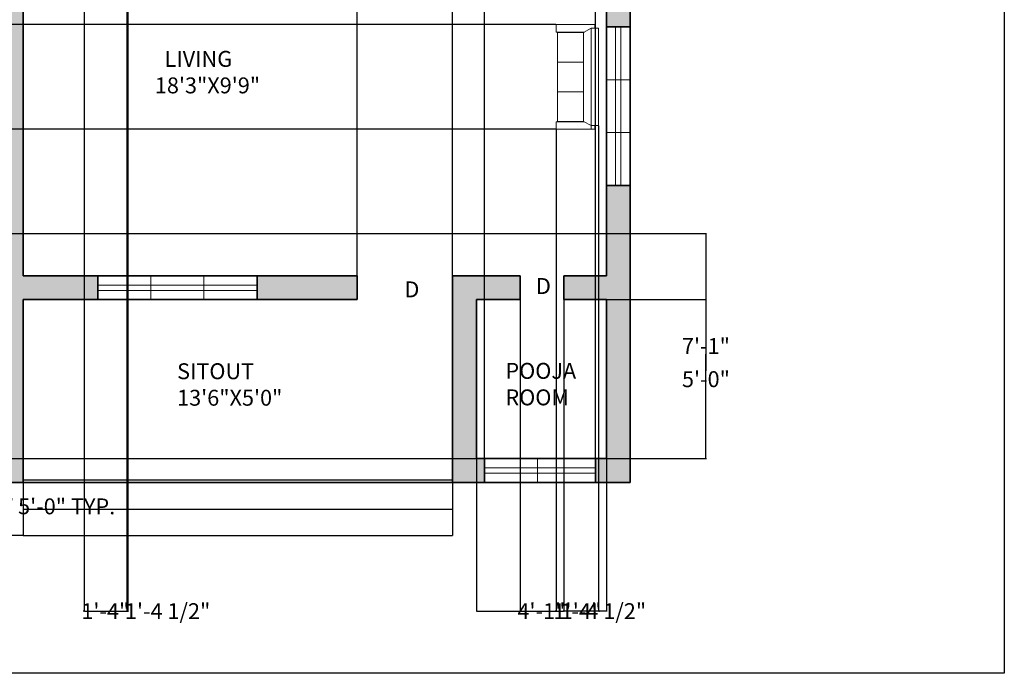
# Model space of a CAD drawing. Units: inches. Extents: x 2552 to 3196, y 4736 to 5443.
# Tile 3 of 8: x 2824 to 3196, y 4736 to 4983. Entities that reach past the tile are written whole.
import ezdxf

# ---------------------------------------------------------------- set-up
doc = ezdxf.new("R2010")
doc.units = ezdxf.units.IN
doc.header["$MEASUREMENT"] = 0
for name, color, linetype, lineweight in [('A-ANNO-DIMS', 2, 'Continuous', 18), ('A-ANNO-TTLB', 7, 'Continuous', 25), ('A-AREA-IDEN', 7, 'Continuous', 18), ('A-DOOR-IDEN', 7, 'Continuous', 18), ('A-FLOR-STRS', 7, 'Continuous', 25), ('A-FURN', 8, 'Continuous', 18), ('A-GLAZ', 4, 'Continuous', 18), ('A-WALL', 7, 'Continuous', 35)]:
    doc.layers.add(name, color=color, linetype=linetype, lineweight=lineweight)
doc.layers.add('A-WALL-PATT', color=30, linetype='Continuous', lineweight=13, true_color=0xf8991e)
doc.styles.get("Standard").update_dxf_attribs({"font": 'arial.ttf'})
doc.dimstyles.get("Standard").update_dxf_attribs({"dimtxt": 6, "dimasz": 0.18, "dimexe": 0.18, "dimexo": 0.0625, "dimgap": 0.09, "dimtad": 0, "dimtih": 1, "dimtoh": 1, "dimdec": 1, "dimzin": 0, "dimdsep": 46, "dimlunit": 3, "dimtxsty": 'Standard', "dimcen": 0.09, "dimadec": 0, "dimazin": 0, "dimtfac": 1, "dimtdec": 1, "dimtofl": 0, "dimtmove": 0, "dimatfit": 3, "dimfxl": 1, "dimtolj": 1, "dimtzin": 0, "dimarcsym": 0})

# ---------------------------------------------------------------- blocks, each defined once
blk = doc.blocks.new('WIN-60IN-THREE-LIGHT')
for p, q in [((60, 9), (0, 9)), ((20, 9), (20, 0)), ((40, 0), (40, 9)), ((60, 5.5), (0, 5.5)), ((0, 3.5), (60, 3.5)), ((0, 0), (60, 0))]:
    blk.add_line(p, q)
blk = doc.blocks.new('*D9')
at = {"layer": 'A-ANNO-DIMS', "color": 0, "lineweight": -2, "transparency": 16777216}
for p, q in [((2725.76, 4808.26), (2725.76, 4799.14)), ((2785.76, 4808.26), (2785.76, 4799.14)), ((2725.94, 4799.32), (2785.58, 4799.32)), ((2785.76, 4799.32), (2785.94, 4799.32))]:
    blk.add_line(p, q, dxfattribs=at)
at = {"layer": 'A-ANNO-DIMS', "color": 0, "transparency": 16777216}
for points in [[(2725.94, 4799.35), (2725.94, 4799.29), (2725.76, 4799.32)], [(2785.58, 4799.35), (2785.58, 4799.29), (2785.76, 4799.32)]]:
    blk.add_solid(points, dxfattribs=at)
at = {"layer": 'Defpoints', "color": 0, "transparency": 16777216}
for p in [(2725.76, 4808.32), (2785.76, 4808.32), (2785.76, 4799.32)]:
    blk.add_point(p, dxfattribs=at)
at = {"layer": 'A-ANNO-DIMS', "color": 0, "transparency": 16777216, "insert": (2823.99, 4799.32), "char_height": 6, "attachment_point": 5}
blk.add_mtext('\\A1;WINDOW 5\'-0" TYP.', dxfattribs=at)
blk = doc.blocks.new('*D21')
at = {"layer": 'A-ANNO-DIMS', "color": 0, "lineweight": -2, "transparency": 16777216}
for p, q in [((2996.66, 4817.26), (2996.66, 4759.59)), ((3045.66, 4817.26), (3045.66, 4759.59)), ((2996.84, 4759.77), (3012.97, 4759.77)), ((3045.48, 4759.77), (3029.34, 4759.77))]:
    blk.add_line(p, q, dxfattribs=at)
at = {"layer": 'A-ANNO-DIMS', "color": 0, "transparency": 16777216}
for points in [[(2996.84, 4759.8), (2996.84, 4759.74), (2996.66, 4759.77)], [(3045.48, 4759.8), (3045.48, 4759.74), (3045.66, 4759.77)]]:
    blk.add_solid(points, dxfattribs=at)
at = {"layer": 'Defpoints', "color": 0, "transparency": 16777216}
for p in [(2996.66, 4817.32), (3045.66, 4817.32), (3045.66, 4759.77)]:
    blk.add_point(p, dxfattribs=at)
at = {"layer": 'A-ANNO-DIMS', "color": 0, "transparency": 16777216, "insert": (3021.16, 4759.77), "char_height": 6, "attachment_point": 5}
blk.add_mtext('\\A1;4\'-1"', dxfattribs=at)
blk = doc.blocks.new('*D22')
at = {"layer": 'A-ANNO-DIMS', "color": 0, "lineweight": -2, "transparency": 16777216}
for p, q in [((3045.72, 4877.32), (3083.39, 4877.32)), ((3083.21, 4877.14), (3083.21, 4850.47)), ((3083.21, 4817.5), (3083.21, 4844.16)), ((3045.72, 4817.32), (3083.39, 4817.32))]:
    blk.add_line(p, q, dxfattribs=at)
at = {"layer": 'A-ANNO-DIMS', "color": 0, "transparency": 16777216}
for points in [[(3083.18, 4877.14), (3083.24, 4877.14), (3083.21, 4877.32)], [(3083.18, 4817.5), (3083.24, 4817.5), (3083.21, 4817.32)]]:
    blk.add_solid(points, dxfattribs=at)
at = {"layer": 'Defpoints', "color": 0, "transparency": 16777216}
for p in [(3045.66, 4877.32), (3083.21, 4877.32), (3045.66, 4817.32)]:
    blk.add_point(p, dxfattribs=at)
at = {"layer": 'A-ANNO-DIMS', "color": 0, "transparency": 16777216, "insert": (3083.21, 4847.32), "char_height": 6, "attachment_point": 5}
blk.add_mtext('\\A1;5\'-0"', dxfattribs=at)
blk = doc.blocks.new('*D23')
at = {"layer": 'A-ANNO-DIMS', "color": 0, "lineweight": -2, "transparency": 16777216}
for p, q in [((2825.59, 4808.32), (2662.93, 4808.32)), ((2663.11, 4808.14), (2663.11, 4801.47)), ((2663.11, 4788.5), (2663.11, 4795.16)), ((2825.59, 4788.32), (2662.93, 4788.32))]:
    blk.add_line(p, q, dxfattribs=at)
at = {"layer": 'A-ANNO-DIMS', "color": 0, "transparency": 16777216}
for points in [[(2663.08, 4808.14), (2663.14, 4808.14), (2663.11, 4808.32)], [(2663.08, 4788.5), (2663.14, 4788.5), (2663.11, 4788.32)]]:
    blk.add_solid(points, dxfattribs=at)
at = {"layer": 'Defpoints', "color": 0, "transparency": 16777216}
for p in [(2663.11, 4808.32), (2825.66, 4808.32), (2825.66, 4788.32)]:
    blk.add_point(p, dxfattribs=at)
at = {"layer": 'A-ANNO-DIMS', "color": 0, "transparency": 16777216, "insert": (2663.11, 4798.32), "char_height": 6, "attachment_point": 5}
blk.add_mtext('\\A1;1\'-8"', dxfattribs=at)
blk = doc.blocks.new('*D24')
at = {"layer": 'A-ANNO-DIMS', "color": 0, "lineweight": -2, "transparency": 16777216}
for p, q in [((2951.66, 4886.38), (2951.66, 5320.05)), ((2951.84, 5319.87), (2961.59, 5319.87)), ((2987.48, 5319.87), (2977.72, 5319.87)), ((2987.66, 4886.38), (2987.66, 5320.05))]:
    blk.add_line(p, q, dxfattribs=at)
at = {"layer": 'A-ANNO-DIMS', "color": 0, "transparency": 16777216}
for points in [[(2951.84, 5319.9), (2951.84, 5319.84), (2951.66, 5319.87)], [(2987.48, 5319.9), (2987.48, 5319.84), (2987.66, 5319.87)]]:
    blk.add_solid(points, dxfattribs=at)
at = {"layer": 'Defpoints', "color": 0, "transparency": 16777216}
for p in [(2987.66, 5319.87), (2951.66, 4886.32), (2987.66, 4886.32)]:
    blk.add_point(p, dxfattribs=at)
at = {"layer": 'A-ANNO-DIMS', "color": 0, "transparency": 16777216, "insert": (2969.66, 5319.87), "char_height": 6, "attachment_point": 5}
blk.add_mtext('\\A1;3\'-0"', dxfattribs=at)
blk = doc.blocks.new('*D25')
at = {"layer": 'A-ANNO-DIMS', "color": 0, "lineweight": -2, "transparency": 16777216}
for p, q in [((3013.11, 4877.26), (3013.11, 4759.59)), ((3029.6, 4877.26), (3029.6, 4759.59)), ((3013.29, 4759.77), (3029.42, 4759.77)), ((3029.6, 4759.77), (3029.78, 4759.77))]:
    blk.add_line(p, q, dxfattribs=at)
at = {"layer": 'A-ANNO-DIMS', "color": 0, "transparency": 16777216}
for points in [[(3013.29, 4759.8), (3013.29, 4759.74), (3013.11, 4759.77)], [(3029.42, 4759.8), (3029.42, 4759.74), (3029.6, 4759.77)]]:
    blk.add_solid(points, dxfattribs=at)
at = {"layer": 'Defpoints', "color": 0, "transparency": 16777216}
for p in [(3013.11, 4877.32), (3029.6, 4877.32), (3029.6, 4759.77)]:
    blk.add_point(p, dxfattribs=at)
at = {"layer": 'A-ANNO-DIMS', "color": 0, "transparency": 16777216, "insert": (3044.56, 4759.77), "char_height": 6, "attachment_point": 5}
blk.add_mtext('\\A1;1\'-4 1/2"', dxfattribs=at)
blk = doc.blocks.new('*D27')
at = {"layer": 'A-ANNO-DIMS', "color": 0, "lineweight": -2, "transparency": 16777216}
for p, q in [((2999.73, 4817.38), (2999.73, 5320.05)), ((2999.91, 5319.87), (3012.6, 5319.87)), ((3041.41, 5319.87), (3028.73, 5319.87)), ((3041.59, 4817.38), (3041.59, 5320.05))]:
    blk.add_line(p, q, dxfattribs=at)
at = {"layer": 'A-ANNO-DIMS', "color": 0, "transparency": 16777216}
for points in [[(2999.91, 5319.9), (2999.91, 5319.84), (2999.73, 5319.87)], [(3041.41, 5319.9), (3041.41, 5319.84), (3041.59, 5319.87)]]:
    blk.add_solid(points, dxfattribs=at)
at = {"layer": 'Defpoints', "color": 0, "transparency": 16777216}
for p in [(3041.59, 5319.87), (2999.73, 4817.32), (3041.59, 4817.32)]:
    blk.add_point(p, dxfattribs=at)
at = {"layer": 'A-ANNO-DIMS', "color": 0, "transparency": 16777216, "insert": (3020.66, 5319.87), "char_height": 6, "attachment_point": 5}
blk.add_mtext('\\A1;3\'-6"', dxfattribs=at)
blk = doc.blocks.new('*D31')
at = {"layer": 'A-ANNO-DIMS', "color": 0, "lineweight": -2, "transparency": 16777216}
for p, q in [((2848.66, 5282.26), (2848.66, 4759.59)), ((2865.22, 5282.26), (2865.22, 4759.59)), ((2848.84, 4759.77), (2865.04, 4759.77)), ((2865.22, 4759.77), (2865.4, 4759.77))]:
    blk.add_line(p, q, dxfattribs=at)
at = {"layer": 'A-ANNO-DIMS', "color": 0, "transparency": 16777216}
for points in [[(2848.84, 4759.8), (2848.84, 4759.74), (2848.66, 4759.77)], [(2865.04, 4759.8), (2865.04, 4759.74), (2865.22, 4759.77)]]:
    blk.add_solid(points, dxfattribs=at)
at = {"layer": 'Defpoints', "color": 0, "transparency": 16777216}
for p in [(2848.66, 5282.32), (2865.22, 5282.32), (2865.22, 4759.77)]:
    blk.add_point(p, dxfattribs=at)
at = {"layer": 'A-ANNO-DIMS', "color": 0, "transparency": 16777216, "insert": (2880.18, 4759.77), "char_height": 6, "attachment_point": 5}
blk.add_mtext('\\A1;1\'-4 1/2"', dxfattribs=at)
blk = doc.blocks.new('*D32')
at = {"layer": 'A-ANNO-DIMS', "color": 0, "lineweight": -2, "transparency": 16777216}
for p, q in [((2864.75, 5194.1), (2864.75, 4759.59)), ((2848.66, 5191.26), (2848.66, 4759.59)), ((2848.48, 4759.77), (2848.3, 4759.77)), ((2864.93, 4759.77), (2865.11, 4759.77))]:
    blk.add_line(p, q, dxfattribs=at)
at = {"layer": 'A-ANNO-DIMS', "color": 0, "transparency": 16777216}
for points in [[(2848.48, 4759.8), (2848.48, 4759.74), (2848.66, 4759.77)], [(2864.93, 4759.8), (2864.93, 4759.74), (2864.75, 4759.77)]]:
    blk.add_solid(points, dxfattribs=at)
at = {"layer": 'Defpoints', "color": 0, "transparency": 16777216}
for p in [(2864.75, 5194.17), (2848.66, 5191.32), (2864.75, 4759.77)]:
    blk.add_point(p, dxfattribs=at)
at = {"layer": 'A-ANNO-DIMS', "color": 0, "transparency": 16777216, "insert": (2856.7, 4759.77), "char_height": 6, "attachment_point": 5}
blk.add_mtext('\\A1;1\'-4"', dxfattribs=at)
blk = doc.blocks.new('*D35')
at = {"layer": 'A-ANNO-DIMS', "color": 0, "lineweight": -2, "transparency": 16777216}
for p, q in [((3026.66, 4981.14), (2662.93, 4981.14)), ((2663.11, 4980.96), (2663.11, 4964.56)), ((2663.11, 4941.78), (2663.11, 4958.17)), ((3026.66, 4941.6), (2662.93, 4941.6))]:
    blk.add_line(p, q, dxfattribs=at)
at = {"layer": 'A-ANNO-DIMS', "color": 0, "transparency": 16777216}
for points in [[(2663.08, 4980.96), (2663.14, 4980.96), (2663.11, 4981.14)], [(2663.08, 4941.78), (2663.14, 4941.78), (2663.11, 4941.6)]]:
    blk.add_solid(points, dxfattribs=at)
at = {"layer": 'Defpoints', "color": 0, "transparency": 16777216}
for p in [(3026.72, 4981.14), (2663.11, 4941.6), (3026.72, 4941.6)]:
    blk.add_point(p, dxfattribs=at)
at = {"layer": 'A-ANNO-DIMS', "color": 0, "transparency": 16777216, "insert": (2663.11, 4961.37), "char_height": 6, "attachment_point": 5}
blk.add_mtext('\\A1;3\'-3 1/2"', dxfattribs=at)
blk = doc.blocks.new('*D36')
at = {"layer": 'A-ANNO-DIMS', "color": 0, "lineweight": -2, "transparency": 16777216}
for p, q in [((3042.69, 4942.94), (3042.69, 4759.59)), ((3026.72, 4941.53), (3026.72, 4759.59)), ((3026.54, 4759.77), (3026.36, 4759.77)), ((3042.87, 4759.77), (3043.05, 4759.77))]:
    blk.add_line(p, q, dxfattribs=at)
at = {"layer": 'A-ANNO-DIMS', "color": 0, "transparency": 16777216}
for points in [[(3026.54, 4759.8), (3026.54, 4759.74), (3026.72, 4759.77)], [(3042.87, 4759.8), (3042.87, 4759.74), (3042.69, 4759.77)]]:
    blk.add_solid(points, dxfattribs=at)
at = {"layer": 'Defpoints', "color": 0, "transparency": 16777216}
for p in [(3042.69, 4943.01), (3026.72, 4941.6), (3042.69, 4759.77)]:
    blk.add_point(p, dxfattribs=at)
at = {"layer": 'A-ANNO-DIMS', "color": 0, "transparency": 16777216, "insert": (3034.7, 4759.77), "char_height": 6, "attachment_point": 5}
blk.add_mtext('\\A1;1\'-4"', dxfattribs=at)
blk = doc.blocks.new('*D39')
at = {"layer": 'A-ANNO-DIMS', "color": 0, "lineweight": -2, "transparency": 16777216}
for p, q in [((2700.72, 4902.32), (3083.39, 4902.32)), ((3083.21, 4902.14), (3083.21, 4862.92)), ((3083.21, 4817.5), (3083.21, 4856.72)), ((2700.72, 4817.32), (3083.39, 4817.32))]:
    blk.add_line(p, q, dxfattribs=at)
at = {"layer": 'A-ANNO-DIMS', "color": 0, "transparency": 16777216}
for points in [[(3083.18, 4902.14), (3083.24, 4902.14), (3083.21, 4902.32)], [(3083.18, 4817.5), (3083.24, 4817.5), (3083.21, 4817.32)]]:
    blk.add_solid(points, dxfattribs=at)
at = {"layer": 'Defpoints', "color": 0, "transparency": 16777216}
for p in [(2700.66, 4902.32), (3083.21, 4902.32), (2700.66, 4817.32)]:
    blk.add_point(p, dxfattribs=at)
at = {"layer": 'A-ANNO-DIMS', "color": 0, "transparency": 16777216, "insert": (3083.21, 4859.82), "char_height": 6, "attachment_point": 5}
blk.add_mtext('\\A1;7\'-1"', dxfattribs=at)

msp = doc.modelspace()

# ---------------------------------------------------------------- hatches: boundary and pattern name
at = {"layer": 'A-WALL-PATT'}
h = msp.add_hatch(color=256, dxfattribs=at)
h.dxf.hatch_style = 1
h.paths.add_polyline_path([(2700.66, 5282.32), (2732.91, 5282.32), (2732.91, 5291.32), (2691.66, 5291.32), (2691.66, 5248.4), (2700.66, 5248.4)])
h.paths.add_polyline_path([(2865.22, 5291.32), (2792.91, 5291.32), (2792.91, 5282.32), (2839.66, 5282.32), (2839.66, 5136.32), (2848.66, 5136.32), (2848.66, 5182.32), (2913.66, 5182.32), (2913.66, 5246.32), (2904.66, 5246.32), (2904.66, 5191.32), (2848.66, 5191.32), (2848.66, 5282.32), (2865.22, 5282.32)])
h.paths.add_polyline_path([(2946.08, 5291.32), (2889.22, 5291.32), (2889.22, 5282.32), (2946.08, 5282.32)])
h.paths.add_polyline_path([(3054.66, 5291.32), (3006.08, 5291.32), (3006.08, 5282.32), (3045.66, 5282.32), (3045.66, 5249.18), (3054.66, 5249.18)])
h.paths.add_polyline_path([(3054.66, 5189.18), (3045.66, 5189.18), (3045.66, 5145.32), (2904.66, 5145.32), (2904.66, 5136.32), (3045.66, 5136.32), (3045.66, 5103.54), (3054.66, 5103.54)])
h.paths.add_polyline_path([(3054.66, 5043.54), (3045.66, 5043.54), (3045.66, 5012.32), (2913.66, 5012.32), (2913.66, 5100.32), (2904.66, 5100.32), (2904.66, 5003.32), (3045.66, 5003.32), (3045.66, 4980.34), (3054.66, 4980.34)])
h.paths.add_polyline_path([(3054.66, 4920.34), (3045.66, 4920.34), (3045.66, 4886.32), (3029.6, 4886.32), (3029.6, 4877.32), (3045.66, 4877.32), (3045.66, 4817.32), (3041.59, 4817.32), (3041.59, 4808.32), (3054.66, 4808.32)])
h.paths.add_polyline_path([(2996.66, 4877.32), (3013.11, 4877.32), (3013.11, 4886.32), (2987.66, 4886.32), (2987.66, 4808.32), (2999.73, 4808.32), (2999.73, 4817.32), (2996.66, 4817.32)])
h.paths.add_polyline_path([(2825.66, 4877.32), (2853.9, 4877.32), (2853.9, 4886.32), (2825.66, 4886.32), (2825.66, 5000.12), (2816.66, 5000.12), (2816.66, 4817.32), (2785.76, 4817.32), (2785.76, 4808.32), (2825.66, 4808.32)])
h.paths.add_polyline_path([(2951.66, 4886.32), (2913.9, 4886.32), (2913.9, 4877.32), (2951.66, 4877.32)])
h.paths.add_polyline_path([(2725.76, 4817.32), (2700.66, 4817.32), (2700.66, 4833.17), (2691.66, 4833.17), (2691.66, 4808.32), (2725.76, 4808.32)])
h.paths.add_polyline_path([(2700.66, 4902.32), (2691.66, 4902.32), (2691.66, 4869.17), (2700.66, 4869.17)])
h.paths.add_polyline_path([(2765.91, 4947.32), (2700.66, 4947.32), (2700.66, 4977.71), (2691.66, 4977.71), (2691.66, 4938.32), (2765.91, 4938.32)])
h.paths.add_polyline_path([(2825.66, 5077.32), (2773.66, 5077.32), (2773.66, 5112.32), (2764.66, 5112.32), (2764.66, 5077.32), (2700.66, 5077.32), (2700.66, 5102.51), (2691.66, 5102.51), (2691.66, 5037.71), (2700.66, 5037.71), (2700.66, 5068.32), (2816.66, 5068.32), (2816.66, 5036.12), (2825.66, 5036.12)])
h.paths.add_polyline_path([(2803.66, 5145.32), (2700.66, 5145.32), (2700.66, 5188.4), (2691.66, 5188.4), (2691.66, 5126.51), (2700.66, 5126.51), (2700.66, 5136.32), (2803.66, 5136.32)])

# ---------------------------------------------------------------- linework, layer by layer
at = {"layer": 'A-ANNO-TTLB'}
msp.add_lwpolyline([(2551.65, 5442.6), (3195.75, 5442.6), (3195.75, 4736.32), (2551.65, 4736.32)], close=True, dxfattribs=at)
at = {"layer": 'A-FLOR-STRS'}
for p, q in [((2825.66, 4809.32), (2987.66, 4809.32)), ((2825.66, 4808.32), (2987.66, 4808.32)), ((2825.66, 4808.32), (2825.66, 4788.32)), ((2987.66, 4808.32), (2987.66, 4788.32)), ((2825.66, 4798.32), (2987.66, 4798.32)), ((2825.66, 4788.32), (2987.66, 4788.32))]:
    msp.add_line(p, q, dxfattribs=at)
at = {"layer": 'A-FURN'}
for p, q in [((3041.28, 4981.14), (3026.72, 4981.14)), ((3026.72, 4978.32), (3026.72, 4981.14)), ((3041.28, 4979.73), (3041.28, 4981.14)), ((3037.45, 4978.32), (3026.72, 4978.32)), ((3037.05, 4978.14), (3039.87, 4979.73)), ((3039.87, 4941.6), (3039.87, 4979.73)), ((3039.87, 4979.73), (3042.69, 4979.73)), ((3042.69, 4943.01), (3042.69, 4979.73)), ((3027.19, 4966.96), (3037.05, 4966.96)), ((3027.19, 4955.78), (3037.05, 4955.78)), ((3037.27, 4944.42), (3026.72, 4944.42)), ((3026.72, 4944.42), (3026.72, 4941.6)), ((3027.19, 4944.59), (3037.05, 4944.59)), ((3039.87, 4943.01), (3037.05, 4944.59)), ((3039.87, 4943.01), (3042.69, 4943.01)), ((3041.28, 4941.6), (3041.28, 4943.01)), ((3041.28, 4941.6), (3026.72, 4941.6))]:
    msp.add_line(p, q, dxfattribs=at)
msp.add_lwpolyline([(3037.05, 4944.59), (3037.05, 4978.14), (3027.19, 4978.14), (3027.19, 4944.59)], dxfattribs=at)
at = {"layer": 'A-GLAZ'}
for p, q in [((2999.73, 4817.32), (3041.59, 4817.32)), ((3019.73, 4808.32), (3019.73, 4817.32)), ((2999.73, 4813.82), (3041.59, 4813.82)), ((3041.59, 4811.82), (2999.73, 4811.82)), ((3041.59, 4808.32), (2999.73, 4808.32))]:
    msp.add_line(p, q, dxfattribs=at)
at = {"layer": 'A-WALL'}
for p, q in [((3054.66, 5291.32), (3054.66, 4808.32)), ((3045.66, 5003.32), (3045.66, 4886.32)), ((2825.66, 5000.12), (2825.66, 4886.32)), ((3045.66, 4980.34), (3054.66, 4980.34)), ((3054.66, 4920.34), (3045.66, 4920.34)), ((2825.66, 4886.32), (2951.66, 4886.32)), ((2853.9, 4886.32), (2853.9, 4877.32)), ((2913.9, 4877.32), (2913.9, 4886.32)), ((2951.66, 4886.32), (2951.66, 4877.32)), ((2987.66, 4886.32), (2987.66, 4808.32)), ((2987.66, 4886.32), (3013.11, 4886.32)), ((3013.11, 4886.32), (3013.11, 4877.32)), ((3029.6, 4877.32), (3029.6, 4886.32)), ((3029.6, 4886.32), (3045.66, 4886.32)), ((2825.66, 4877.32), (2951.66, 4877.32)), ((2825.66, 4877.32), (2825.66, 4808.32)), ((2996.66, 4877.32), (2996.66, 4817.32)), ((2996.66, 4877.32), (3013.11, 4877.32)), ((3029.6, 4877.32), (3045.66, 4877.32)), ((3045.66, 4877.32), (3045.66, 4817.32)), ((2996.66, 4817.32), (3045.66, 4817.32)), ((2999.73, 4808.32), (2999.73, 4817.32)), ((3041.59, 4817.32), (3041.59, 4808.32)), ((2691.66, 4808.32), (3054.66, 4808.32))]:
    msp.add_line(p, q, dxfattribs=at)

# ---------------------------------------------------------------- block references
at = {"layer": 'A-GLAZ', "rotation": 89.99999999999903}
msp.add_blockref('WIN-60IN-THREE-LIGHT', (3054.66, 4920.34), dxfattribs=at)
at = {"layer": 'A-GLAZ'}
msp.add_blockref('WIN-60IN-THREE-LIGHT', (2853.9, 4877.32), dxfattribs=at)

# ---------------------------------------------------------------- texts
at = {"layer": 'A-AREA-IDEN', "char_height": 6, "attachment_point": 1}
for s, width, insert in [('  LIVING\\P18\'3"X9\'9"', 111.7207, (2875.36, 4971.18)), ('SITOUT\\P13\'6"X5\'0"', 93.2404, (2883.75, 4853.31)), ('POOJA\\PROOM', 44.4868, (3007.58, 4853.45))]:
    msp.add_mtext_dynamic_manual_height_columns(s, width=width, gutter_width=1, heights=[0], dxfattribs=dict(at, insert=insert))
at = {"layer": 'A-DOOR-IDEN', "char_height": 6, "attachment_point": 1}
for insert in [(2969.49, 4884.2), (3019.11, 4885.47)]:
    msp.add_mtext_dynamic_manual_height_columns('D', width=10.2167, gutter_width=1, heights=[0], dxfattribs=dict(at, insert=insert))

# ---------------------------------------------------------------- dimensions: what is measured, and where the dimension line sits
at = {"layer": 'A-ANNO-DIMS'}
for base, p1, p2, picture, middle in [((2987.66, 5319.87), (2951.66, 4886.32), (2987.66, 4886.32), '*D24', (2969.66, 5319.87)), ((3041.59, 5319.87), (2999.73, 4817.32), (3041.59, 4817.32), '*D27', (3020.66, 5319.87)), ((2865.22, 4759.77), (2848.66, 5282.32), (2865.22, 5282.32), '*D31', (2880.18, 4759.77)), ((2864.75, 4759.77), (2848.66, 5191.32), (2864.75, 5194.17), '*D32', (2856.7, 4759.77)), ((3042.69, 4759.77), (3026.72, 4941.6), (3042.69, 4943.01), '*D36', (3034.7, 4759.77)), ((3029.6, 4759.77), (3013.11, 4877.32), (3029.6, 4877.32), '*D25', (3044.56, 4759.77)), ((3045.66, 4759.77), (2996.66, 4817.32), (3045.66, 4817.32), '*D21', (3021.16, 4759.77))]:
    dim = msp.add_linear_dim(base=base, p1=p1, p2=p2, dimstyle='Standard', override={"dimdec": 1, "dimlfac": 1, "dimrnd": 0, "dimzin": 1, "dimdsep": 46, "dimlunit": 4, "dimfrac": 2}, dxfattribs=at)
    dim.commit()
    dim.dimension.update_dxf_attribs({"geometry": picture, "text_midpoint": middle})
for base, p1, p2, picture, middle in [((2663.11, 4941.6), (3026.72, 4981.14), (3026.72, 4941.6), '*D35', (2663.11, 4961.37)), ((3083.21, 4902.32), (2700.66, 4817.32), (2700.66, 4902.32), '*D39', (3083.21, 4859.82)), ((3083.21, 4877.32), (3045.66, 4817.32), (3045.66, 4877.32), '*D22', (3083.21, 4847.32)), ((2663.11, 4808.32), (2825.66, 4788.32), (2825.66, 4808.32), '*D23', (2663.11, 4798.32))]:
    dim = msp.add_linear_dim(base=base, p1=p1, p2=p2, angle=90, dimstyle='Standard', override={"dimdec": 1, "dimlfac": 1, "dimrnd": 0, "dimzin": 1, "dimdsep": 46, "dimlunit": 4, "dimfrac": 2}, dxfattribs=at)
    dim.commit()
    dim.dimension.update_dxf_attribs({"geometry": picture, "text_midpoint": middle})
dim = msp.add_linear_dim(base=(2785.76, 4799.32), p1=(2725.76, 4808.32), p2=(2785.76, 4808.32), text='WINDOW <> TYP.', dimstyle='Standard', override={"dimdec": 1, "dimlfac": 1, "dimrnd": 0, "dimzin": 1, "dimdsep": 46, "dimlunit": 4, "dimfrac": 2}, dxfattribs=at)
dim.commit()
dim.dimension.update_dxf_attribs({"geometry": '*D9', "text_midpoint": (2823.99, 4799.32)})

doc.saveas('drawing.dxf')
